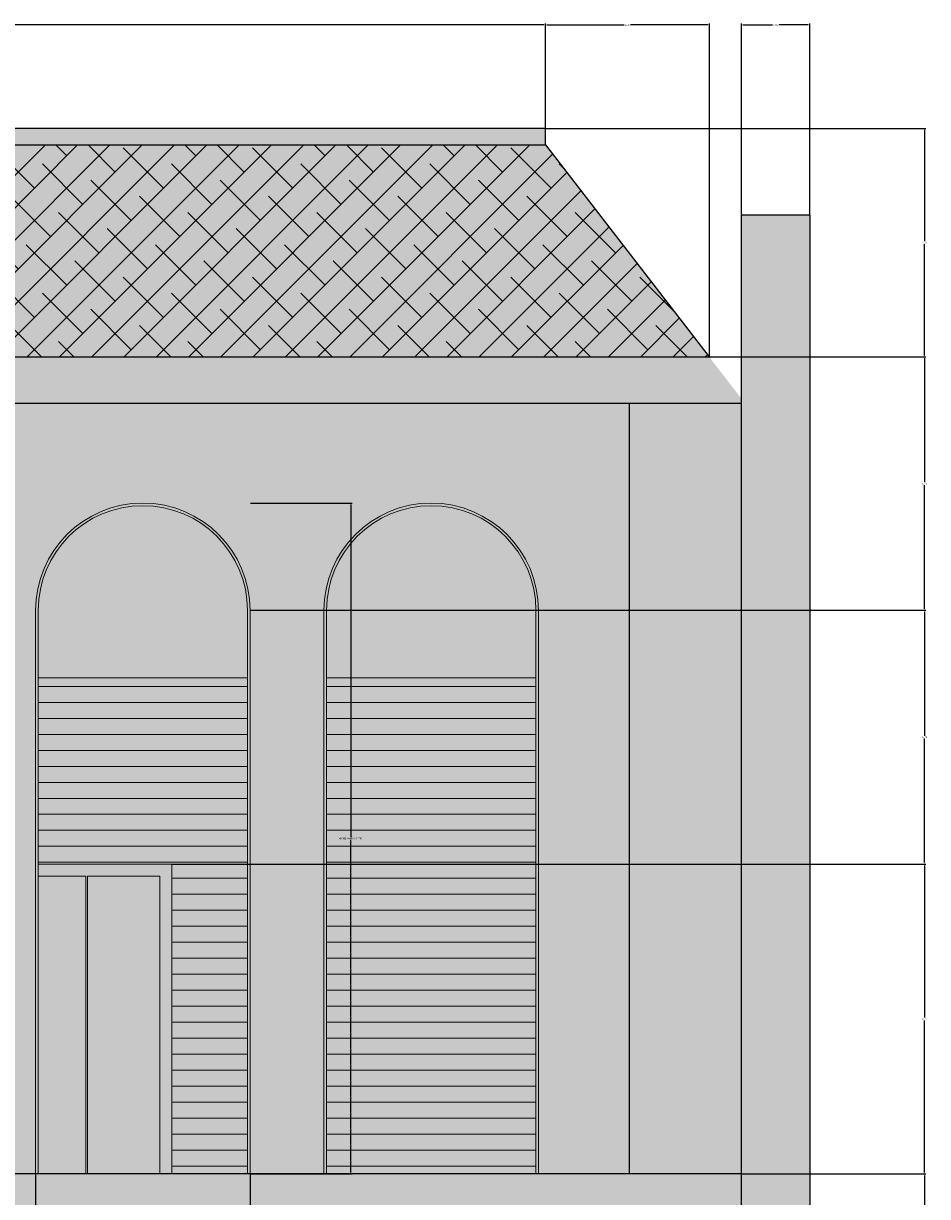
# Model space of a CAD drawing. Units: feet. Extents: x 2352 to 2983, y 950 to 1233.
# Tile 3 of 5: x 2504 to 2617, y 1086 to 1233. Entities that reach past the tile are written whole.
import ezdxf

# ---------------------------------------------------------------- set-up
doc = ezdxf.new("R2010")
doc.units = ezdxf.units.FT
for name, color, linetype, lineweight in [('A-ANNO-DIMS', 2, 'Continuous', 18), ('A-ELEV', 7, 'Continuous', 25), ('A-ELEV-PATT', 252, 'Continuous', 13), ('A-GLAZ', 4, 'Continuous', 18)]:
    doc.layers.add(name, color=color, linetype=linetype, lineweight=lineweight)
doc.styles.get("Standard").update_dxf_attribs({"font": 'arial.ttf'})
doc.dimstyles.get("Standard").update_dxf_attribs({"dimtxt": 0.18, "dimasz": 0.18, "dimexe": 0.18, "dimexo": 0.0625, "dimgap": 0.09, "dimtad": 0, "dimtih": 1, "dimtoh": 1, "dimdec": 1, "dimzin": 0, "dimdsep": 46, "dimlunit": 3, "dimtxsty": 'Standard', "dimcen": 0.09, "dimadec": 0, "dimazin": 0, "dimtfac": 1, "dimtdec": 1, "dimtofl": 0, "dimtmove": 0, "dimatfit": 3, "dimfxl": 1, "dimtolj": 1, "dimtzin": 0, "dimarcsym": 0})

# ---------------------------------------------------------------- blocks, each defined once
blk = doc.blocks.new('WIN-ARCH')
blk.add_line((0.33, 62.05), (26.52, 62.05))
blk.add_line((0.33, 62.05), (26.52, 62.05))
blk.add_lwpolyline([(0, 0), (0, 70.51, -1), (26.84, 70.51), (26.84, 0)], format="xyb")
blk.add_lwpolyline([(0, 0), (0, 70.51, -1), (26.84, 70.51), (26.84, 0)], format="xyb")
blk.add_lwpolyline([(26.52, 70.51), (26.52, 0), (0.33, 0), (0.33, 70.51, -1)], format="xyb", close=True)
blk.add_lwpolyline([(26.52, 70.51), (26.52, 0), (0.33, 0), (0.33, 70.51, -1)], format="xyb", close=True)
blk = doc.blocks.new('*D3')
at = {"layer": 'A-ANNO-DIMS', "color": 0, "lineweight": -2, "transparency": 16777216}
for p, q in [((2532.55, 1172.95), (2545.26, 1172.95)), ((2545.08, 1172.77), (2545.08, 1131.16)), ((2545.08, 1089.19), (2545.08, 1130.8)), ((2532.55, 1089.01), (2545.26, 1089.01))]:
    blk.add_line(p, q, dxfattribs=at)
at = {"layer": 'A-ANNO-DIMS', "color": 0, "transparency": 16777216}
for points in [[(2545.05, 1172.77), (2545.11, 1172.77), (2545.08, 1172.95)], [(2545.05, 1089.19), (2545.11, 1089.19), (2545.08, 1089.01)]]:
    blk.add_solid(points, dxfattribs=at)
at = {"layer": 'Defpoints', "color": 0, "transparency": 16777216}
for p in [(2532.49, 1172.95), (2545.08, 1172.95), (2532.49, 1089.01)]:
    blk.add_point(p, dxfattribs=at)
at = {"layer": 'A-ANNO-DIMS', "color": 0, "transparency": 16777216, "insert": (2545.08, 1130.98), "char_height": 0.18, "attachment_point": 5}
blk.add_mtext('\\A1;ARCHED WINDOW 84 TYP.', dxfattribs=at)
blk = doc.blocks.new('*D4')
at = {"layer": 'A-ANNO-DIMS', "color": 0, "lineweight": -2, "transparency": 16777216}
for p, q in [((2505.64, 1088.95), (2505.64, 1076.24)), ((2532.49, 1088.95), (2532.49, 1076.24)), ((2505.82, 1076.42), (2518.53, 1076.42)), ((2532.31, 1076.42), (2519.59, 1076.42))]:
    blk.add_line(p, q, dxfattribs=at)
at = {"layer": 'A-ANNO-DIMS', "color": 0, "transparency": 16777216}
for points in [[(2505.82, 1076.45), (2505.82, 1076.39), (2505.64, 1076.42)], [(2532.31, 1076.45), (2532.31, 1076.39), (2532.49, 1076.42)]]:
    blk.add_solid(points, dxfattribs=at)
at = {"layer": 'Defpoints', "color": 0, "transparency": 16777216}
for p in [(2505.64, 1089.01), (2532.49, 1089.01), (2532.49, 1076.42)]:
    blk.add_point(p, dxfattribs=at)
at = {"layer": 'A-ANNO-DIMS', "color": 0, "transparency": 16777216, "insert": (2519.06, 1076.42), "char_height": 0.18, "attachment_point": 5}
blk.add_mtext('\\A1;27 TYP.', dxfattribs=at)
blk = doc.blocks.new('*D9')
at = {"layer": 'A-ANNO-DIMS', "color": 0, "lineweight": -2, "transparency": 16777216}
for p, q in [((2403.34, 1219.88), (2403.34, 1232.95)), ((2569.44, 1219.88), (2569.44, 1232.95)), ((2403.52, 1232.77), (2486.02, 1232.77)), ((2569.26, 1232.77), (2486.76, 1232.77))]:
    blk.add_line(p, q, dxfattribs=at)
at = {"layer": 'A-ANNO-DIMS', "color": 0, "transparency": 16777216}
for points in [[(2403.52, 1232.8), (2403.52, 1232.74), (2403.34, 1232.77)], [(2569.26, 1232.8), (2569.26, 1232.74), (2569.44, 1232.77)]]:
    blk.add_solid(points, dxfattribs=at)
at = {"layer": 'Defpoints', "color": 0, "transparency": 16777216}
for p in [(2569.44, 1232.77), (2403.34, 1219.82), (2569.44, 1219.82)]:
    blk.add_point(p, dxfattribs=at)
at = {"layer": 'A-ANNO-DIMS', "color": 0, "transparency": 16777216, "insert": (2486.39, 1232.77), "char_height": 0.18, "attachment_point": 5}
blk.add_mtext('\\A1;166.1', dxfattribs=at)
blk = doc.blocks.new('*D10')
at = {"layer": 'A-ANNO-DIMS', "color": 0, "lineweight": -2, "transparency": 16777216}
for p, q in [((2569.44, 1217.81), (2569.44, 1232.95)), ((2589.97, 1191.25), (2589.97, 1232.95)), ((2569.62, 1232.77), (2579.31, 1232.77)), ((2589.79, 1232.77), (2580.1, 1232.77))]:
    blk.add_line(p, q, dxfattribs=at)
at = {"layer": 'A-ANNO-DIMS', "color": 0, "transparency": 16777216}
for points in [[(2569.62, 1232.8), (2569.62, 1232.74), (2569.44, 1232.77)], [(2589.79, 1232.8), (2589.79, 1232.74), (2589.97, 1232.77)]]:
    blk.add_solid(points, dxfattribs=at)
at = {"layer": 'Defpoints', "color": 0, "transparency": 16777216}
for p in [(2589.97, 1232.77), (2569.44, 1217.75), (2589.97, 1191.19)]:
    blk.add_point(p, dxfattribs=at)
at = {"layer": 'A-ANNO-DIMS', "color": 0, "transparency": 16777216, "insert": (2579.71, 1232.77), "char_height": 0.18, "attachment_point": 5}
blk.add_mtext('\\A1;20.53', dxfattribs=at)
blk = doc.blocks.new('*D11')
at = {"layer": 'A-ANNO-DIMS', "color": 0, "lineweight": -2, "transparency": 16777216}
for p, q in [((2593.97, 1209.08), (2593.97, 1232.95)), ((2602.53, 1209.08), (2602.53, 1232.95)), ((2594.15, 1232.77), (2597.85, 1232.77)), ((2602.35, 1232.77), (2598.64, 1232.77))]:
    blk.add_line(p, q, dxfattribs=at)
at = {"layer": 'A-ANNO-DIMS', "color": 0, "transparency": 16777216}
for points in [[(2594.15, 1232.8), (2594.15, 1232.74), (2593.97, 1232.77)], [(2602.35, 1232.8), (2602.35, 1232.74), (2602.53, 1232.77)]]:
    blk.add_solid(points, dxfattribs=at)
at = {"layer": 'Defpoints', "color": 0, "transparency": 16777216}
for p in [(2602.53, 1232.77), (2593.97, 1209.01), (2602.53, 1209.01)]:
    blk.add_point(p, dxfattribs=at)
at = {"layer": 'A-ANNO-DIMS', "color": 0, "transparency": 16777216, "insert": (2598.25, 1232.77), "char_height": 0.18, "attachment_point": 5}
blk.add_mtext('\\A1;8.562', dxfattribs=at)
blk = doc.blocks.new('*D17')
at = {"layer": 'A-ANNO-DIMS', "color": 0, "lineweight": -2, "transparency": 16777216}
for p, q in [((2594.03, 1089.01), (2617.07, 1089.01)), ((2616.89, 1088.83), (2616.89, 1082.75)), ((2616.89, 1076.3), (2616.89, 1082.38)), ((2594.03, 1076.12), (2617.07, 1076.12))]:
    blk.add_line(p, q, dxfattribs=at)
at = {"layer": 'A-ANNO-DIMS', "color": 0, "transparency": 16777216}
for points in [[(2616.86, 1088.83), (2616.92, 1088.83), (2616.89, 1089.01)], [(2616.86, 1076.3), (2616.92, 1076.3), (2616.89, 1076.12)]]:
    blk.add_solid(points, dxfattribs=at)
at = {"layer": 'Defpoints', "color": 0, "transparency": 16777216}
for p in [(2593.97, 1089.01), (2616.89, 1089.01), (2593.97, 1076.12)]:
    blk.add_point(p, dxfattribs=at)
at = {"layer": 'A-ANNO-DIMS', "color": 0, "transparency": 16777216, "insert": (2616.89, 1082.57), "char_height": 0.18, "attachment_point": 5}
blk.add_mtext('\\A1;12.892', dxfattribs=at)
blk = doc.blocks.new('*D18')
at = {"layer": 'A-ANNO-DIMS', "color": 0, "lineweight": -2, "transparency": 16777216}
for p, q in [((2522.75, 1127.78), (2617.07, 1127.78)), ((2616.89, 1127.6), (2616.89, 1108.58)), ((2616.89, 1089.19), (2616.89, 1108.21)), ((2594.03, 1089.01), (2617.07, 1089.01))]:
    blk.add_line(p, q, dxfattribs=at)
at = {"layer": 'A-ANNO-DIMS', "color": 0, "transparency": 16777216}
for points in [[(2616.86, 1127.6), (2616.92, 1127.6), (2616.89, 1127.78)], [(2616.86, 1089.19), (2616.92, 1089.19), (2616.89, 1089.01)]]:
    blk.add_solid(points, dxfattribs=at)
at = {"layer": 'Defpoints', "color": 0, "transparency": 16777216}
for p in [(2522.69, 1127.78), (2616.89, 1127.78), (2593.97, 1089.01)]:
    blk.add_point(p, dxfattribs=at)
at = {"layer": 'A-ANNO-DIMS', "color": 0, "transparency": 16777216, "insert": (2616.89, 1108.4), "char_height": 0.18, "attachment_point": 5}
blk.add_mtext('\\A1;38.77', dxfattribs=at)
blk = doc.blocks.new('*D19')
at = {"layer": 'A-ANNO-DIMS', "color": 0, "lineweight": -2, "transparency": 16777216}
for p, q in [((2532.55, 1159.53), (2617.07, 1159.53)), ((2616.89, 1159.35), (2616.89, 1143.84)), ((2616.89, 1127.96), (2616.89, 1143.47)), ((2522.75, 1127.78), (2617.07, 1127.78))]:
    blk.add_line(p, q, dxfattribs=at)
at = {"layer": 'A-ANNO-DIMS', "color": 0, "transparency": 16777216}
for points in [[(2616.86, 1159.35), (2616.92, 1159.35), (2616.89, 1159.53)], [(2616.86, 1127.96), (2616.92, 1127.96), (2616.89, 1127.78)]]:
    blk.add_solid(points, dxfattribs=at)
at = {"layer": 'Defpoints', "color": 0, "transparency": 16777216}
for p in [(2532.49, 1159.53), (2616.89, 1159.53), (2522.69, 1127.78)]:
    blk.add_point(p, dxfattribs=at)
at = {"layer": 'A-ANNO-DIMS', "color": 0, "transparency": 16777216, "insert": (2616.89, 1143.65), "char_height": 0.18, "attachment_point": 5}
blk.add_mtext('\\A1;31.75', dxfattribs=at)
blk = doc.blocks.new('*D20')
at = {"layer": 'A-ANNO-DIMS', "color": 0, "lineweight": -2, "transparency": 16777216}
for p, q in [((2594.03, 1191.24), (2617.07, 1191.24)), ((2616.89, 1191.06), (2616.89, 1175.56)), ((2616.89, 1159.71), (2616.89, 1175.2)), ((2532.55, 1159.53), (2617.07, 1159.53))]:
    blk.add_line(p, q, dxfattribs=at)
at = {"layer": 'A-ANNO-DIMS', "color": 0, "transparency": 16777216}
for points in [[(2616.86, 1191.06), (2616.92, 1191.06), (2616.89, 1191.24)], [(2616.86, 1159.71), (2616.92, 1159.71), (2616.89, 1159.53)]]:
    blk.add_solid(points, dxfattribs=at)
at = {"layer": 'Defpoints', "color": 0, "transparency": 16777216}
for p in [(2593.97, 1191.24), (2616.89, 1191.24), (2532.49, 1159.53)]:
    blk.add_point(p, dxfattribs=at)
at = {"layer": 'A-ANNO-DIMS', "color": 0, "transparency": 16777216, "insert": (2616.89, 1175.38), "char_height": 0.18, "attachment_point": 5}
blk.add_mtext('\\A1;31.71', dxfattribs=at)
blk = doc.blocks.new('*D21')
at = {"layer": 'A-ANNO-DIMS', "color": 0, "lineweight": -2, "transparency": 16777216}
for p, q in [((2569.5, 1219.82), (2617.07, 1219.82)), ((2616.89, 1219.64), (2616.89, 1205.71)), ((2616.89, 1191.42), (2616.89, 1205.35)), ((2594.03, 1191.24), (2617.07, 1191.24))]:
    blk.add_line(p, q, dxfattribs=at)
at = {"layer": 'A-ANNO-DIMS', "color": 0, "transparency": 16777216}
for points in [[(2616.86, 1219.64), (2616.92, 1219.64), (2616.89, 1219.82)], [(2616.86, 1191.42), (2616.92, 1191.42), (2616.89, 1191.24)]]:
    blk.add_solid(points, dxfattribs=at)
at = {"layer": 'Defpoints', "color": 0, "transparency": 16777216}
for p in [(2569.44, 1219.82), (2616.89, 1219.82), (2593.97, 1191.24)]:
    blk.add_point(p, dxfattribs=at)
at = {"layer": 'A-ANNO-DIMS', "color": 0, "transparency": 16777216, "insert": (2616.89, 1205.53), "char_height": 0.18, "attachment_point": 5}
blk.add_mtext('\\A1;28.58', dxfattribs=at)

msp = doc.modelspace()

# ---------------------------------------------------------------- hatches: boundary and pattern name
at = {"layer": 'A-ELEV-PATT'}
h = msp.add_hatch(color=256, dxfattribs=at)
h.dxf.hatch_style = 1
h.paths.add_polyline_path([(2499.5465, 1215.0126), (2373.2965, 1215.0126), (2373.2965, 1209.0126), (2499.5465, 1209.0126)])
h.paths.add_polyline_path([(2502.6085, 1217.7513), (2403.3368, 1217.7513), (2373.2965, 1217.7513), (2373.2965, 1215.0126), (2499.5465, 1215.0126)])
h.paths.add_polyline_path([(2569.4416, 1219.8182), (2403.3368, 1219.8182), (2403.3368, 1217.7513), (2569.4416, 1217.7513)])
h.paths.add_polyline_path([(2593.9663, 1076.1207), (2582.4111, 1069.3398), (2582.4111, 1011.4831), (2595.2079, 1011.4831), (2595.2079, 1023.0126), (2594.1881, 1024.8551), (2594.1881, 1026.3357), (2594.1891, 1026.3338, 0.10932946), (2593.9663, 1027.4578)])
h.paths.add_polyline_path([(2602.5286, 1209.0126), (2593.9663, 1209.0126), (2593.9663, 1027.4578), (2595.2079, 1025.2146), (2602.5286, 1025.2146)])
h.paths.add_polyline_path([(2593.9663, 1083.0126), (2497.3422, 1083.0126), (2497.3422, 1076.1207), (2593.9663, 1076.1207)])
h.paths.add_polyline_path([(2485.8114, 1075.3288), (2384.8273, 1075.3288), (2384.8273, 1011.4831), (2398.2572, 1011.4831), (2398.2572, 1042.4514), (2479.5304, 1042.4514), (2479.5304, 1025.2146), (2485.8114, 1025.2146)])
h.paths.add_polyline_path([(2485.8114, 1083.0126), (2383.4779, 1083.0126), (2383.4779, 1076.1207), (2485.8114, 1076.1207)])
h.paths.add_polyline_path([(2495.9928, 1089.0126), (2491.6239, 1089.0126), (2491.6239, 1025.2146), (2495.9928, 1025.2146)])
h.paths.add_polyline_path([(2491.5297, 1089.0126), (2488.0105, 1089.0126), (2488.0105, 1025.2146), (2491.5297, 1025.2146)])
h.paths.add_polyline_path([(2379.0148, 1129.0147), (2375.4956, 1129.0147), (2375.4956, 1025.2146), (2379.0148, 1025.2146)])
h.paths.add_polyline_path([(2383.4779, 1129.0147), (2379.109, 1129.0147), (2379.109, 1025.2146), (2381.1604, 1025.2146), (2383.4779, 1025.8769)])
h.paths.add_polyline_path([(2389.4076, 1144.6653), (2389.4076, 1142.2389), (2384.8273, 1142.2389), (2384.8273, 1089.0126), (2397.2412, 1089.0126), (2397.2412, 1156.1636), (2471.8066, 1156.1636), (2471.8066, 1089.0126), (2485.8114, 1089.0126), (2485.8114, 1142.2389), (2480.0884, 1142.2389), (2480.0884, 1144.6653, 0.80625477)])
h.paths.add_polyline_path([(2389.4076, 1144.6653, -0.80625477), (2480.0884, 1144.6653, 1)])
h.paths.add_polyline_path([(2579.9743, 1185.4477), (2497.3422, 1185.4477), (2497.3422, 1147.0918), (2498.0576, 1146.9764), (2497.8725, 1144.5798, 0.11184527), (2497.3422, 1142.5724), (2497.3422, 1089.0126), (2505.6415, 1089.0126), (2505.6415, 1159.528, -1), (2532.4859, 1159.528), (2532.4859, 1089.0126), (2541.7346, 1089.0126), (2541.7346, 1159.528, -1), (2568.579, 1159.528), (2568.579, 1089.0126), (2579.9743, 1089.0126)])
h.paths.add_polyline_path([(2579.9743, 1191.2362), (2497.3422, 1191.2362), (2497.3422, 1185.4477), (2579.9743, 1185.4477)])
h.paths.add_polyline_path([(2381.1604, 1023.0126), (2367.0741, 1023.0126), (2367.0741, 963.0126), (2381.1604, 963.0126)])
h.paths.add_polyline_path([(2495.2282, 1011.4831), (2495.2282, 1023.0126), (2439.9479, 1023.0126), (2439.9479, 963.0126), (2446.428, 963.0126), (2446.428, 989.9926, -1), (2485.4222, 989.9926), (2485.4222, 963.0126), (2495.2282, 963.0126)])
h.paths.add_polyline_path([(2446.428, 989.9926), (2446.428, 963.0126), (2485.4222, 963.0126), (2485.4222, 989.9926, 1)], flags=17)
h.paths.add_polyline_path([(2603.7702, 1023.0126), (2595.2079, 1023.0126), (2595.2079, 1011.4831), (2595.2079, 963.0126), (2603.7702, 963.0126)])
h.paths.add_polyline_path([(2482.4531, 1147.0918), (2497.3422, 1147.0918), (2497.3422, 1185.4477), (2497.3422, 1194.3715), (2373.2965, 1194.3715), (2373.2965, 1147.0918), (2387.0428, 1147.0918, -0.95042953)])
h.paths.add_polyline_path([(2384.8273, 1142.2389), (2373.2965, 1142.2389), (2373.2965, 1129.0147), (2384.8273, 1129.0147)])
h.paths.add_polyline_path([(2495.9928, 1142.2389), (2488.0105, 1142.2389), (2488.0105, 1089.0126), (2491.5297, 1089.0126), (2495.9928, 1089.0126)])
h = msp.add_hatch(color=256, dxfattribs=at)
h.dxf.hatch_style = 1
h.paths.add_polyline_path([(2595.2079, 1011.4831), (2495.2282, 1011.4831), (2495.2282, 963.0126), (2595.2079, 963.0126)])
h.paths.add_polyline_path([(2579.9743, 1204.1231), (2569.4416, 1217.7513), (2502.6085, 1217.7513), (2499.5465, 1215.0126), (2499.5465, 1209.0126), (2497.3422, 1209.0126), (2497.3422, 1195.936), (2498.0772, 1195.936), (2498.0772, 1195.1775), (2497.8022, 1194.3715), (2497.3422, 1194.3715), (2497.3422, 1191.2362), (2579.9743, 1191.2362)])
h = msp.add_hatch(dxfattribs=at)
h.set_pattern_fill('ANSI38', color=256, scale=0.9)
h.paths.add_polyline_path([(2569.4416, 1217.7513), (2502.6085, 1217.7513), (2499.5465, 1215.0126), (2499.5465, 1209.0126), (2497.3422, 1209.0126), (2497.3422, 1195.936), (2498.0772, 1195.936), (2498.0772, 1195.1775), (2497.8022, 1194.3715), (2497.3422, 1194.3715), (2497.3422, 1191.2362), (2579.9743, 1191.2362), (2579.9743, 1204.1231)])
h.paths.add_polyline_path([(2579.9743, 1204.1231), (2579.9743, 1191.2362), (2589.9732, 1191.1856)])
h = msp.add_hatch(color=256, dxfattribs=at)
h.dxf.hatch_style = 1
h.paths.add_polyline_path([(2579.9743, 1204.1231), (2579.9743, 1191.2362), (2589.9732, 1191.1856)])
h = msp.add_hatch(color=256, dxfattribs=at)
h.dxf.hatch_style = 1
h.paths.add_polyline_path([(2480.0884, 1144.6653), (2497.3422, 1144.6653), (2497.8725, 1144.5798), (2498.0576, 1146.9764), (2497.3422, 1147.0918), (2482.4531, 1147.0918, 0.95042953), (2387.0428, 1147.0918), (2373.2965, 1147.0918), (2371.8622, 1147.0918), (2372.5793, 1144.6653), (2389.4076, 1144.6653, -1)])
h.paths.add_polyline_path([(2389.4076, 1144.6653), (2372.5793, 1144.6653), (2373.2965, 1142.2389), (2389.4076, 1142.2389)])
h.paths.add_polyline_path([(2497.8725, 1144.5798), (2497.3422, 1144.6653), (2480.0884, 1144.6653), (2480.0884, 1142.2389), (2497.3422, 1142.2389, -0.12985075)])
h.paths.add_polyline_path([(2471.8066, 1156.1636), (2397.2412, 1156.1636), (2397.2412, 1089.0126), (2398.6146, 1089.0126), (2398.6146, 1154.7902), (2470.4332, 1154.7902), (2470.4332, 1089.0126), (2471.8066, 1089.0126)])
h.paths.add_polyline_path([(2470.4332, 1154.7902), (2398.6146, 1154.7902), (2398.6146, 1089.0126), (2400.114, 1089.0126), (2400.114, 1153.2908), (2468.9338, 1153.2908), (2468.9338, 1089.0126), (2470.4332, 1089.0126)], flags=17)
h.paths.add_polyline_path([(2495.8508, 1024.4932), (2439.2183, 1024.4932), (2439.2183, 1023.0126), (2495.8508, 1023.0126)])
h.paths.add_polyline_path([(2496.3417, 1025.2146), (2438.7275, 1025.2146, -0.22451739), (2439.2183, 1024.4932), (2495.8508, 1024.4932, -0.22451739)])
h.paths.add_polyline_path([(2381.1604, 1024.4932), (2366.1676, 1024.4932), (2366.1676, 1023.0126), (2381.1604, 1023.0126)])
h.paths.add_polyline_path([(2381.1604, 1025.2146), (2365.4325, 1025.2146, -0.12196493), (2366.1676, 1024.4932), (2381.1604, 1024.4932)])
h.paths.add_polyline_path([(2383.4779, 1025.1555), (2383.4779, 1025.8769), (2381.1604, 1025.2146), (2381.1604, 1024.4932)])
h.paths.add_polyline_path([(2383.4779, 1025.1555), (2381.1604, 1024.4932), (2381.1604, 1023.0126), (2383.4779, 1023.6749)])
h.paths.add_polyline_path([(2479.5304, 1042.4514), (2398.2572, 1042.4514), (2398.2572, 1011.4831), (2399.3703, 1011.4831), (2399.3703, 1041.3383), (2478.4174, 1041.3383), (2478.4174, 1025.2146), (2479.5304, 1025.2146)])
h.paths.add_polyline_path([(2478.4174, 1041.3383), (2399.3703, 1041.3383), (2399.3703, 1011.4831), (2400.6982, 1011.4831), (2400.6982, 1040.0104), (2477.0895, 1040.0104), (2477.0895, 1025.2146), (2478.4174, 1025.2146)], flags=17)
h.paths.add_polyline_path([(2565.0085, 1048.4289), (2535.3542, 1048.4289), (2535.3542, 1011.4831), (2536.3698, 1011.4831), (2536.3698, 1047.4133), (2563.993, 1047.4133), (2563.993, 1011.4831), (2565.0085, 1011.4831)])
h.paths.add_polyline_path([(2522.2926, 1048.4289), (2497.3422, 1048.4289), (2497.3422, 1047.4929), (2521.3566, 1047.4929), (2521.3566, 1011.4831), (2522.2926, 1011.4831)])
h.paths.add_polyline_path([(2603.9449, 1025.2146), (2603.7702, 1025.2146), (2595.2079, 1025.2146), (2593.9663, 1027.4578, -0.10932946), (2594.1891, 1026.3338), (2595.2079, 1024.4932), (2603.7702, 1024.4932, -0.10758073)])
h.paths.add_polyline_path([(2603.7702, 1024.4932), (2595.2079, 1024.4932), (2594.1891, 1026.3338, -0.00342101), (2594.1881, 1026.2975), (2594.1881, 1024.8551), (2595.2079, 1023.0126), (2603.7702, 1023.0126)])
h.paths.add_polyline_path([(2532.4859, 1159.528, 1), (2505.6415, 1159.528), (2505.6415, 1089.0126), (2505.9696, 1089.0126), (2505.9696, 1126.273), (2505.9696, 1159.528, -1), (2532.1578, 1159.528), (2532.1578, 1089.0126), (2532.4859, 1089.0126)])
h.paths.add_polyline_path([(2542.0627, 1159.528, -1), (2568.2509, 1159.528), (2568.2509, 1089.0126), (2568.579, 1089.0126), (2568.579, 1159.528, 1), (2541.7346, 1159.528), (2541.7346, 1089.0126), (2542.0627, 1089.0126)])
h.paths.add_polyline_path([(2522.687, 1127.7792), (2505.9696, 1127.7792), (2505.9696, 1126.273), (2511.9257, 1126.273), (2511.9257, 1089.0126), (2512.1488, 1089.0126), (2512.1488, 1126.273), (2521.1808, 1126.273), (2521.1808, 1089.0126), (2522.687, 1089.0126)], flags=17)
h.paths.add_polyline_path([(2439.9479, 1011.4831), (2381.1604, 1011.4831), (2381.1604, 963.0126), (2439.9479, 963.0126)])
h = msp.add_hatch(color=256, dxfattribs=at)
h.dxf.hatch_style = 1
h.paths.add_polyline_path([(2589.9732, 1191.1856), (2579.9743, 1191.2362), (2579.9743, 1185.4477), (2593.9663, 1185.4477), (2593.9663, 1186.0189)])
h.paths.add_polyline_path([(2593.9663, 1185.4477), (2579.9743, 1185.4477), (2579.9743, 1089.0126), (2593.9663, 1089.0126)])
h = msp.add_hatch(color=256, dxfattribs=at)
h.dxf.hatch_style = 1
h.paths.add_polyline_path([(2582.4111, 1069.3398), (2497.3422, 1069.3398), (2497.3422, 1048.4289), (2522.2926, 1048.4289), (2522.2926, 1011.4831), (2535.3542, 1011.4831), (2535.3542, 1048.4289), (2565.0085, 1048.4289), (2565.0085, 1011.4831), (2582.4111, 1011.4831)])
h.paths.add_polyline_path([(2568.2509, 1151.0596), (2542.0627, 1151.0596), (2542.0627, 1089.0126), (2568.2509, 1089.0126)])
h.paths.add_polyline_path([(2532.1578, 1151.0596), (2505.9696, 1151.0596), (2505.9696, 1127.7792), (2522.687, 1127.7792), (2522.687, 1089.0126), (2532.1578, 1089.0126)])
h.paths.add_polyline_path([(2505.9696, 1159.528), (2505.9696, 1151.0596), (2532.1578, 1151.0596), (2532.1578, 1159.528, 1)])
h.paths.add_polyline_path([(2568.2509, 1159.528, 1), (2542.0627, 1159.528), (2542.0627, 1151.0596), (2568.2509, 1151.0596)])
h = msp.add_hatch(dxfattribs=at)
h.set_pattern_fill('_USER', color=256, scale=2, pattern_type=0)
h.set_pattern_definition([(0, (0, 0), (0, 2), [])])
h.paths.add_polyline_path([(2532.1578, 1151.0596), (2505.9696, 1151.0596), (2505.9696, 1127.7792), (2522.687, 1127.7792), (2522.687, 1089.0126), (2532.1578, 1089.0126)])
h.paths.add_polyline_path([(2568.2509, 1151.0596), (2542.0627, 1151.0596), (2542.0627, 1089.0126), (2568.2509, 1089.0126)])
h.paths.add_polyline_path([(2582.4111, 1069.3398), (2497.3422, 1069.3398), (2497.3422, 1048.4289), (2522.2926, 1048.4289), (2522.2926, 1011.4831), (2535.3542, 1011.4831), (2535.3542, 1048.4289), (2565.0085, 1048.4289), (2565.0085, 1011.4831), (2582.4111, 1011.4831)])
h = msp.add_hatch(color=256, dxfattribs=at)
h.dxf.hatch_style = 1
h.paths.add_polyline_path([(2438.1858, 1039.4184), (2401.2902, 1039.4184), (2401.2902, 1011.4831), (2438.1858, 1011.4831)])
h.paths.add_polyline_path([(2476.4975, 1039.4184), (2440.2408, 1039.4184), (2440.2408, 1025.2146), (2476.4975, 1025.2146)])
h.paths.add_polyline_path([(2563.252, 1046.6724), (2550.43, 1046.6724), (2550.43, 1011.4831), (2563.252, 1011.4831)])
h.paths.add_polyline_path([(2549.9328, 1046.6724), (2537.1107, 1046.6724), (2537.1107, 1011.4831), (2549.9328, 1011.4831)])
h.paths.add_polyline_path([(2520.4416, 1046.5779), (2507.7848, 1046.5779), (2507.7848, 1011.4831), (2520.4416, 1011.4831)])
h.paths.add_polyline_path([(2506.8593, 1046.5779), (2497.3422, 1046.5779), (2497.3422, 1011.4831), (2506.8593, 1011.4831)])
h.paths.add_polyline_path([(2521.1808, 1126.273), (2512.1488, 1126.273), (2512.1488, 1089.0126), (2521.1808, 1089.0126)])
h.paths.add_polyline_path([(2511.9257, 1126.273), (2505.9696, 1126.273), (2505.9696, 1089.0126), (2511.9257, 1089.0126)])
h.paths.add_polyline_path([(2466.1883, 1150.5453), (2435.4142, 1150.5453), (2435.4142, 1089.0126), (2466.1883, 1089.0126)])
h.paths.add_polyline_path([(2433.6336, 1150.5453), (2402.8595, 1150.5453), (2402.8595, 1089.0126), (2433.6336, 1089.0126)])
h = msp.add_hatch(color=256, dxfattribs=at)
h.dxf.hatch_style = 1
h.paths.add_polyline_path([(2593.9663, 1089.0126), (2497.3422, 1089.0126), (2497.3422, 1083.0126), (2593.9663, 1083.0126)])
h.paths.add_polyline_path([(2485.8114, 1089.0126), (2384.8273, 1089.0126), (2384.8273, 1083.0126), (2485.8114, 1083.0126)])
h.paths.add_polyline_path([(2375.4956, 1129.0147), (2373.2965, 1129.0147), (2373.2965, 1025.2146), (2375.4956, 1025.2146)])
h.paths.add_polyline_path([(2384.8273, 1129.0147), (2383.4779, 1129.0147), (2383.4779, 1083.0126), (2384.8273, 1083.0126)])
h.paths.add_polyline_path([(2384.8273, 1075.3288), (2383.4779, 1076.1207), (2383.4779, 1025.8769), (2383.4779, 1011.4831), (2384.8273, 1011.4831)])
h.paths.add_polyline_path([(2488.0105, 1089.0126), (2485.8114, 1089.0126), (2485.8114, 1025.2146), (2488.0105, 1025.2146)])
h.paths.add_polyline_path([(2497.3422, 1089.0126), (2495.9928, 1089.0126), (2495.9928, 1025.2146), (2496.3417, 1025.2146, 0.22451739), (2495.8508, 1024.4932), (2495.8508, 1023.0126), (2495.2282, 1023.0126), (2495.2282, 1011.4831), (2497.3422, 1011.4831), (2497.3422, 1048.4289)])
h.paths.add_polyline_path([(2497.3422, 1142.2389), (2495.9928, 1142.2389), (2495.9928, 1089.0126), (2497.3422, 1089.0126)])
h.paths.add_polyline_path([(2488.0105, 1142.2389), (2485.8114, 1142.2389), (2485.8114, 1089.0126), (2488.0105, 1089.0126)])

# ---------------------------------------------------------------- linework, layer by layer
at = {"layer": 'A-ELEV'}
for p, q in [((2569.4416, 1217.7513), (2589.9341, 1191.2362)), ((2593.9663, 1209.0126), (2602.5286, 1209.0126)), ((2593.9663, 1209.0126), (2602.5286, 1209.0126)), ((2497.3422, 1191.2362), (2579.9743, 1191.2362)), ((2497.3422, 1191.2362), (2589.9341, 1191.2362)), ((2579.9743, 1191.2362), (2589.9732, 1191.1856)), ((2589.9341, 1191.2362), (2593.9663, 1191.2362)), ((2497.3422, 1185.4477), (2593.9663, 1185.4477)), ((2579.9743, 1089.0126), (2579.9743, 1185.4477)), ((2579.9743, 1185.4477), (2593.9663, 1185.4477)), ((2593.9663, 1089.0126), (2497.3422, 1089.0126)), ((2593.9663, 1089.0126), (2497.3422, 1089.0126))]:
    msp.add_line(p, q, dxfattribs=at)
msp.add_lwpolyline([(2403.3368, 1217.7513), (2569.4416, 1217.7513), (2569.4416, 1219.8182), (2403.3368, 1219.8182)], close=True, dxfattribs=at)
msp.add_lwpolyline([(2403.3368, 1217.7513), (2569.4416, 1217.7513), (2569.4416, 1219.8182), (2403.3368, 1219.8182)], close=True, dxfattribs=at)
for points in [[(2593.9663, 1027.4578), (2593.9663, 1209.0126)], [(2593.9663, 1027.4578), (2593.9663, 1209.0126)], [(2602.5286, 1209.0126), (2602.5286, 1025.2146), (2595.2079, 1025.2146)], [(2602.5286, 1209.0126), (2602.5286, 1025.2146), (2595.2079, 1025.2146)]]:
    msp.add_lwpolyline(points, dxfattribs=at)
at = {"layer": 'A-GLAZ'}
for points in [[(2522.687, 1089.0126), (2522.687, 1127.7792), (2505.9696, 1127.7792)], [(2522.687, 1089.0126), (2522.687, 1127.7792), (2505.9696, 1127.7792)], [(2511.9257, 1126.273), (2505.9696, 1126.273), (2505.9696, 1089.0126), (2521.1808, 1089.0126), (2521.1808, 1126.273), (2512.1488, 1126.273)], [(2511.9257, 1126.273), (2505.9696, 1126.273), (2505.9696, 1089.0126), (2521.1808, 1089.0126), (2521.1808, 1126.273), (2512.1488, 1126.273)], [(2512.1488, 1126.273), (2512.1488, 1089.0126), (2511.9257, 1089.0126), (2511.9257, 1126.273)], [(2512.1488, 1126.273), (2512.1488, 1089.0126), (2511.9257, 1089.0126), (2511.9257, 1126.273)]]:
    msp.add_lwpolyline(points, dxfattribs=at)

# ---------------------------------------------------------------- block references
for p in [(2505.642, 1089.013), (2541.7351, 1089.013)]:
    msp.add_blockref('WIN-ARCH', p, dxfattribs=at)

# ---------------------------------------------------------------- dimensions: what is measured, and where the dimension line sits
at = {"layer": 'A-ANNO-DIMS'}
for base, p1, p2, override, picture, middle in [((2569.4416, 1232.7682), (2403.3368, 1219.8182), (2569.4416, 1219.8182), {"dimdec": 1, "dimlfac": 1, "dimrnd": 0, "dimzin": 0, "dimdsep": 46, "dimlunit": 2}, '*D9', (2486.3892, 1232.7682)), ((2589.9732, 1232.7682), (2569.4416, 1217.7513), (2589.9732, 1191.1856), {"dimdec": 2, "dimlfac": 1, "dimrnd": 0, "dimzin": 0, "dimdsep": 46, "dimlunit": 2}, '*D10', (2579.7074, 1232.7682)), ((2602.5286, 1232.7682), (2593.9663, 1209.0126), (2602.5286, 1209.0126), {"dimdec": 3, "dimlfac": 1, "dimrnd": 0, "dimzin": 0, "dimdsep": 46, "dimlunit": 2}, '*D11', (2598.2474, 1232.7682))]:
    dim = msp.add_linear_dim(base=base, p1=p1, p2=p2, dimstyle='Standard', override=override, dxfattribs=at)
    dim.commit()
    dim.dimension.update_dxf_attribs({"geometry": picture, "text_midpoint": middle})
for base, p1, p2, override, picture, middle in [((2616.8949, 1219.8182), (2593.9663, 1191.2362), (2569.4416, 1219.8182), {"dimdec": 2, "dimlfac": 1, "dimrnd": 0, "dimzin": 0, "dimdsep": 46, "dimlunit": 2}, '*D21', (2616.8949, 1205.5272)), ((2616.8949, 1191.2362), (2532.4859, 1159.528), (2593.9663, 1191.2362), {"dimdec": 2, "dimlfac": 1, "dimrnd": 0, "dimzin": 0, "dimdsep": 46, "dimlunit": 2}, '*D20', (2616.8949, 1175.3821)), ((2616.8949, 1159.528), (2522.687, 1127.7792), (2532.4859, 1159.528), {"dimdec": 2, "dimlfac": 1, "dimrnd": 0, "dimzin": 0, "dimdsep": 46, "dimlunit": 2}, '*D19', (2616.8949, 1143.6536)), ((2616.8949, 1127.7792), (2593.9663, 1089.0126), (2522.687, 1127.7792), {"dimdec": 2, "dimlfac": 1, "dimrnd": 0, "dimzin": 0, "dimdsep": 46, "dimlunit": 2}, '*D18', (2616.8949, 1108.3959)), ((2616.8949, 1089.0126), (2593.9663, 1076.1207), (2593.9663, 1089.0126), {"dimdec": 3, "dimlfac": 1, "dimrnd": 0, "dimzin": 0, "dimdsep": 46, "dimlunit": 2}, '*D17', (2616.8949, 1082.5667))]:
    dim = msp.add_linear_dim(base=base, p1=p1, p2=p2, angle=90, dimstyle='Standard', override=override, dxfattribs=at)
    dim.commit()
    dim.dimension.update_dxf_attribs({"geometry": picture, "text_midpoint": middle})
dim = msp.add_linear_dim(base=(2545.0766, 1172.9502), p1=(2532.4859, 1089.0126), p2=(2532.4859, 1172.9502), angle=90, text='ARCHED WINDOW <> TYP.', dimstyle='Standard', override={"dimdec": 0, "dimrnd": 0, "dimzin": 0, "dimlunit": 2}, dxfattribs=at)
dim.commit()
dim.dimension.update_dxf_attribs({"geometry": '*D3', "text_midpoint": (2545.0766, 1130.9814)})
dim = msp.add_linear_dim(base=(2532.4859, 1076.422), p1=(2505.6415, 1089.0126), p2=(2532.4859, 1089.0126), text='<> TYP.', dimstyle='Standard', override={"dimdec": 0, "dimrnd": 0, "dimzin": 0, "dimlunit": 2}, dxfattribs=at)
dim.commit()
dim.dimension.update_dxf_attribs({"geometry": '*D4', "text_midpoint": (2519.0637, 1076.422)})

doc.saveas('drawing.dxf')
